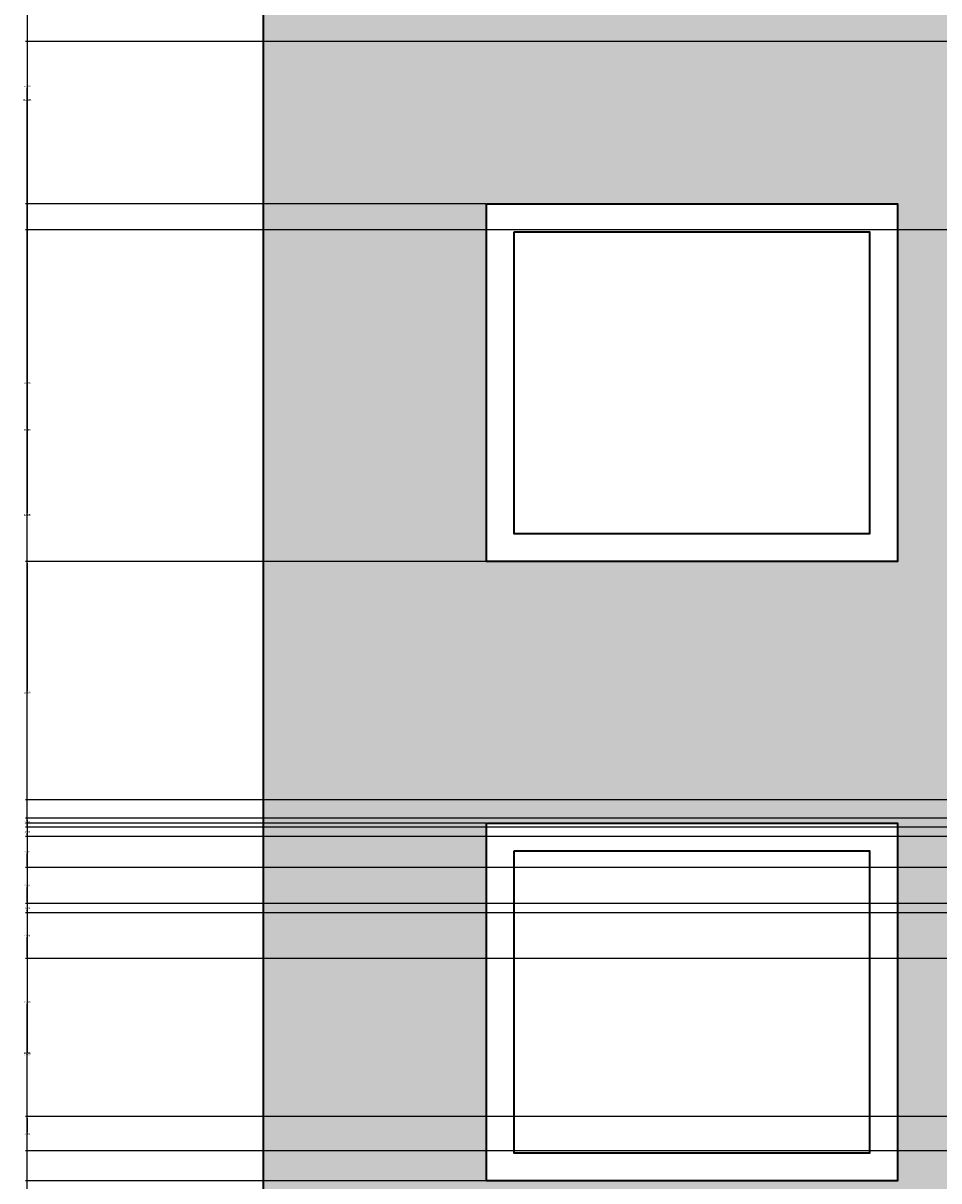
# Model space of a CAD drawing. Units: inches. Extents: x 93 to 565, y 123 to 656.
# Tile 5 of 18: x 93 to 192, y 324 to 450. Entities that reach past the tile are written whole.
import ezdxf

# ---------------------------------------------------------------- set-up
doc = ezdxf.new("R2010")
doc.units = ezdxf.units.IN
doc.header["$MEASUREMENT"] = 0
for name, color, linetype, lineweight in [('A-ANNO-DIMS', 2, 'Continuous', 18), ('A-ELEV', 7, 'Continuous', 35), ('A-WALL-PATT', 8, 'Continuous', 13)]:
    doc.layers.add(name, color=color, linetype=linetype, lineweight=lineweight)
doc.styles.get("Standard").update_dxf_attribs({"font": 'arial.ttf'})
doc.dimstyles.get("Standard").update_dxf_attribs({"dimtxt": 0.18, "dimasz": 0.18, "dimexe": 0.18, "dimexo": 0.0625, "dimgap": 0.09, "dimtad": 0, "dimtih": 1, "dimtoh": 1, "dimdec": 4, "dimzin": 0, "dimdsep": 46, "dimtxsty": 'Standard', "dimcen": 0.09, "dimadec": 0, "dimazin": 0, "dimtfac": 1, "dimtdec": 4, "dimtofl": 0, "dimtmove": 0, "dimatfit": 3, "dimfxl": 1, "dimtolj": 1, "dimtzin": 0, "dimarcsym": 0})

# ---------------------------------------------------------------- blocks, each defined once
blk = doc.blocks.new('*D27')
at = {"layer": 'A-ANNO-DIMS', "color": 0, "lineweight": -2, "transparency": 16777216}
for p, q in [((210.54, 519.04), (210.54, 134)), ((119.08, 159.67), (119.08, 134)), ((119.26, 134.18), (164.42, 134.18)), ((210.36, 134.18), (165.21, 134.18))]:
    blk.add_line(p, q, dxfattribs=at)
at = {"layer": 'A-ANNO-DIMS', "color": 0, "transparency": 16777216}
for points in [[(119.26, 134.21), (119.26, 134.15), (119.08, 134.18)], [(210.36, 134.21), (210.36, 134.15), (210.54, 134.18)]]:
    blk.add_solid(points, dxfattribs=at)
at = {"layer": 'Defpoints', "color": 0, "transparency": 16777216}
for p in [(210.54, 519.1), (119.08, 159.73), (210.54, 134.18)]:
    blk.add_point(p, dxfattribs=at)
at = {"layer": 'A-ANNO-DIMS', "color": 0, "transparency": 16777216, "insert": (164.81, 134.18), "char_height": 0.18, "attachment_point": 5}
blk.add_mtext('\\A1;91.46', dxfattribs=at)
blk = doc.blocks.new('*D31')
at = {"layer": 'A-ANNO-DIMS', "color": 0, "lineweight": -2, "transparency": 16777216}
for p, q in [((417.87, 630.4), (564.81, 630.4)), ((564.63, 630.22), (564.63, 395.25)), ((564.63, 159.91), (564.63, 394.89)), ((119.14, 159.73), (564.81, 159.73))]:
    blk.add_line(p, q, dxfattribs=at)
at = {"layer": 'A-ANNO-DIMS', "color": 0, "transparency": 16777216}
for points in [[(564.6, 630.22), (564.66, 630.22), (564.63, 630.4)], [(564.6, 159.91), (564.66, 159.91), (564.63, 159.73)]]:
    blk.add_solid(points, dxfattribs=at)
at = {"layer": 'Defpoints', "color": 0, "transparency": 16777216}
for p in [(417.81, 630.4), (564.63, 630.4), (119.08, 159.73)]:
    blk.add_point(p, dxfattribs=at)
at = {"layer": 'A-ANNO-DIMS', "color": 0, "transparency": 16777216, "insert": (564.63, 395.07), "char_height": 0.18, "attachment_point": 5}
blk.add_mtext('\\A1;470.7', dxfattribs=at)
blk = doc.blocks.new('*D34')
at = {"layer": 'A-ANNO-DIMS', "color": 0, "lineweight": -2, "transparency": 16777216}
for p, q in [((286.62, 363.73), (93.35, 363.73)), ((93.53, 363.55), (93.53, 338.52)), ((93.53, 313.13), (93.53, 338.16)), ((286.62, 312.95), (93.35, 312.95))]:
    blk.add_line(p, q, dxfattribs=at)
at = {"layer": 'A-ANNO-DIMS', "color": 0, "transparency": 16777216}
for points in [[(93.5, 363.55), (93.56, 363.55), (93.53, 363.73)], [(93.5, 313.13), (93.56, 313.13), (93.53, 312.95)]]:
    blk.add_solid(points, dxfattribs=at)
at = {"layer": 'Defpoints', "color": 0, "transparency": 16777216}
for p in [(93.53, 363.73), (286.69, 363.73), (286.69, 312.95)]:
    blk.add_point(p, dxfattribs=at)
at = {"layer": 'A-ANNO-DIMS', "color": 0, "transparency": 16777216, "insert": (93.53, 338.34), "char_height": 0.18, "attachment_point": 5}
blk.add_mtext('\\A1;50.78', dxfattribs=at)
blk = doc.blocks.new('*D35')
at = {"layer": 'A-ANNO-DIMS', "color": 0, "lineweight": -2, "transparency": 16777216}
for p, q in [((119.02, 519.1), (93.35, 519.1)), ((93.53, 518.92), (93.53, 441.6)), ((93.53, 363.91), (93.53, 441.23)), ((286.62, 363.73), (93.35, 363.73))]:
    blk.add_line(p, q, dxfattribs=at)
at = {"layer": 'A-ANNO-DIMS', "color": 0, "transparency": 16777216}
for points in [[(93.5, 518.92), (93.56, 518.92), (93.53, 519.1)], [(93.5, 363.91), (93.56, 363.91), (93.53, 363.73)]]:
    blk.add_solid(points, dxfattribs=at)
at = {"layer": 'Defpoints', "color": 0, "transparency": 16777216}
for p in [(93.53, 519.1), (119.08, 519.1), (286.69, 363.73)]:
    blk.add_point(p, dxfattribs=at)
at = {"layer": 'A-ANNO-DIMS', "color": 0, "transparency": 16777216, "insert": (93.53, 441.42), "char_height": 0.18, "attachment_point": 5}
blk.add_mtext('\\A1;155.37', dxfattribs=at)
blk = doc.blocks.new('*D43')
at = {"layer": 'A-ANNO-DIMS', "color": 0, "lineweight": -2, "transparency": 16777216}
for p, q in [((143.15, 363.17), (93.35, 363.17)), ((93.53, 362.99), (93.53, 344.01)), ((93.53, 324.67), (93.53, 343.65)), ((143.15, 324.49), (93.35, 324.49))]:
    blk.add_line(p, q, dxfattribs=at)
at = {"layer": 'A-ANNO-DIMS', "color": 0, "transparency": 16777216}
for points in [[(93.5, 362.99), (93.56, 362.99), (93.53, 363.17)], [(93.5, 324.67), (93.56, 324.67), (93.53, 324.49)]]:
    blk.add_solid(points, dxfattribs=at)
at = {"layer": 'Defpoints', "color": 0, "transparency": 16777216}
for p in [(93.53, 363.17), (143.21, 363.17), (143.21, 324.49)]:
    blk.add_point(p, dxfattribs=at)
at = {"layer": 'A-ANNO-DIMS', "color": 0, "transparency": 16777216, "insert": (93.53, 343.83), "char_height": 0.18, "attachment_point": 5}
blk.add_mtext('\\A1;38.685', dxfattribs=at)
blk = doc.blocks.new('*D44')
at = {"layer": 'A-ANNO-DIMS', "color": 0, "lineweight": -2, "transparency": 16777216}
for p, q in [((143.15, 391.47), (93.35, 391.47)), ((93.53, 391.29), (93.53, 377.5)), ((93.53, 363.35), (93.53, 377.14)), ((143.15, 363.17), (93.35, 363.17))]:
    blk.add_line(p, q, dxfattribs=at)
at = {"layer": 'A-ANNO-DIMS', "color": 0, "transparency": 16777216}
for points in [[(93.5, 391.29), (93.56, 391.29), (93.53, 391.47)], [(93.5, 363.35), (93.56, 363.35), (93.53, 363.17)]]:
    blk.add_solid(points, dxfattribs=at)
at = {"layer": 'Defpoints', "color": 0, "transparency": 16777216}
for p in [(93.53, 391.47), (143.21, 391.47), (143.21, 363.17)]:
    blk.add_point(p, dxfattribs=at)
at = {"layer": 'A-ANNO-DIMS', "color": 0, "transparency": 16777216, "insert": (93.53, 377.32), "char_height": 0.18, "attachment_point": 5}
blk.add_mtext('\\A1;28.295', dxfattribs=at)
blk = doc.blocks.new('*D45')
at = {"layer": 'A-ANNO-DIMS', "color": 0, "lineweight": -2, "transparency": 16777216}
for p, q in [((143.15, 430.15), (93.35, 430.15)), ((93.53, 429.97), (93.53, 410.99)), ((93.53, 391.65), (93.53, 410.63)), ((143.15, 391.47), (93.35, 391.47))]:
    blk.add_line(p, q, dxfattribs=at)
at = {"layer": 'A-ANNO-DIMS', "color": 0, "transparency": 16777216}
for points in [[(93.5, 429.97), (93.56, 429.97), (93.53, 430.15)], [(93.5, 391.65), (93.56, 391.65), (93.53, 391.47)]]:
    blk.add_solid(points, dxfattribs=at)
at = {"layer": 'Defpoints', "color": 0, "transparency": 16777216}
for p in [(93.53, 430.15), (143.21, 430.15), (143.21, 391.47)]:
    blk.add_point(p, dxfattribs=at)
at = {"layer": 'A-ANNO-DIMS', "color": 0, "transparency": 16777216, "insert": (93.53, 410.81), "char_height": 0.18, "attachment_point": 5}
blk.add_mtext('\\A1;38.685', dxfattribs=at)
blk = doc.blocks.new('*D46')
at = {"layer": 'A-ANNO-DIMS', "color": 0, "lineweight": -2, "transparency": 16777216}
for p, q in [((143.15, 455.66), (93.35, 455.66)), ((93.53, 455.48), (93.53, 443.09)), ((93.53, 430.33), (93.53, 442.72)), ((143.15, 430.15), (93.35, 430.15))]:
    blk.add_line(p, q, dxfattribs=at)
at = {"layer": 'A-ANNO-DIMS', "color": 0, "transparency": 16777216}
for points in [[(93.5, 455.48), (93.56, 455.48), (93.53, 455.66)], [(93.5, 430.33), (93.56, 430.33), (93.53, 430.15)]]:
    blk.add_solid(points, dxfattribs=at)
at = {"layer": 'Defpoints', "color": 0, "transparency": 16777216}
for p in [(93.53, 455.66), (143.21, 455.66), (143.21, 430.15)]:
    blk.add_point(p, dxfattribs=at)
at = {"layer": 'A-ANNO-DIMS', "color": 0, "transparency": 16777216, "insert": (93.53, 442.9), "char_height": 0.18, "attachment_point": 5}
blk.add_mtext('\\A1;25.507', dxfattribs=at)
blk = doc.blocks.new('*D65')
at = {"layer": 'A-ANNO-DIMS', "color": 0, "lineweight": -2, "transparency": 16777216}
for p, q in [((265.15, 427.35), (93.35, 427.35)), ((93.53, 427.17), (93.53, 396.71)), ((93.53, 365.89), (93.53, 396.35)), ((262.24, 365.71), (93.35, 365.71))]:
    blk.add_line(p, q, dxfattribs=at)
at = {"layer": 'A-ANNO-DIMS', "color": 0, "transparency": 16777216}
for points in [[(93.5, 427.17), (93.56, 427.17), (93.53, 427.35)], [(93.5, 365.89), (93.56, 365.89), (93.53, 365.71)]]:
    blk.add_solid(points, dxfattribs=at)
at = {"layer": 'Defpoints', "color": 0, "transparency": 16777216}
for p in [(93.53, 427.35), (265.21, 427.35), (262.3, 365.71)]:
    blk.add_point(p, dxfattribs=at)
at = {"layer": 'A-ANNO-DIMS', "color": 0, "transparency": 16777216, "insert": (93.53, 396.53), "char_height": 0.18, "attachment_point": 5}
blk.add_mtext('\\A1;61.64', dxfattribs=at)
blk = doc.blocks.new('*D72')
at = {"layer": 'A-ANNO-DIMS', "color": 0, "lineweight": -2, "transparency": 16777216}
for p, q in [((295.62, 447.73), (93.35, 447.73)), ((93.53, 447.55), (93.53, 405.91)), ((93.53, 363.91), (93.53, 405.55)), ((286.62, 363.73), (93.35, 363.73))]:
    blk.add_line(p, q, dxfattribs=at)
at = {"layer": 'A-ANNO-DIMS', "color": 0, "transparency": 16777216}
for points in [[(93.5, 447.55), (93.56, 447.55), (93.53, 447.73)], [(93.5, 363.91), (93.56, 363.91), (93.53, 363.73)]]:
    blk.add_solid(points, dxfattribs=at)
at = {"layer": 'Defpoints', "color": 0, "transparency": 16777216}
for p in [(295.69, 447.73), (93.53, 363.73), (286.69, 363.73)]:
    blk.add_point(p, dxfattribs=at)
at = {"layer": 'A-ANNO-DIMS', "color": 0, "transparency": 16777216, "insert": (93.53, 405.73), "char_height": 0.18, "attachment_point": 5}
blk.add_mtext('\\A1;84', dxfattribs=at)
blk = doc.blocks.new('*D106')
at = {"layer": 'A-ANNO-DIMS', "color": 0, "lineweight": -2, "transparency": 16777216}
for p, q in [((210.54, 519.04), (210.54, 134)), ((119.08, 159.67), (119.08, 134)), ((119.26, 134.18), (164.35, 134.18)), ((210.36, 134.18), (165.28, 134.18))]:
    blk.add_line(p, q, dxfattribs=at)
at = {"layer": 'A-ANNO-DIMS', "color": 0, "transparency": 16777216}
for points in [[(119.26, 134.21), (119.26, 134.15), (119.08, 134.18)], [(210.36, 134.21), (210.36, 134.15), (210.54, 134.18)]]:
    blk.add_solid(points, dxfattribs=at)
at = {"layer": 'Defpoints', "color": 0, "transparency": 16777216}
for p in [(210.54, 519.1), (119.08, 159.73), (210.54, 134.18)]:
    blk.add_point(p, dxfattribs=at)
at = {"layer": 'A-ANNO-DIMS', "color": 0, "transparency": 16777216, "insert": (164.81, 134.18), "char_height": 0.18, "attachment_point": 5}
blk.add_mtext('\\A1;91.465', dxfattribs=at)
blk = doc.blocks.new('*D110')
at = {"layer": 'A-ANNO-DIMS', "color": 0, "lineweight": -2, "transparency": 16777216}
for p, q in [((417.87, 630.4), (564.81, 630.4)), ((564.63, 630.22), (564.63, 395.25)), ((564.63, 159.91), (564.63, 394.89)), ((119.14, 159.73), (564.81, 159.73))]:
    blk.add_line(p, q, dxfattribs=at)
at = {"layer": 'A-ANNO-DIMS', "color": 0, "transparency": 16777216}
for points in [[(564.6, 630.22), (564.66, 630.22), (564.63, 630.4)], [(564.6, 159.91), (564.66, 159.91), (564.63, 159.73)]]:
    blk.add_solid(points, dxfattribs=at)
at = {"layer": 'Defpoints', "color": 0, "transparency": 16777216}
for p in [(417.81, 630.4), (564.63, 630.4), (119.08, 159.73)]:
    blk.add_point(p, dxfattribs=at)
at = {"layer": 'A-ANNO-DIMS', "color": 0, "transparency": 16777216, "insert": (564.63, 395.07), "char_height": 0.18, "attachment_point": 5}
blk.add_mtext('\\A1;470.673', dxfattribs=at)
blk = doc.blocks.new('*D113')
at = {"layer": 'A-ANNO-DIMS', "color": 0, "lineweight": -2, "transparency": 16777216}
for p, q in [((286.62, 363.73), (93.35, 363.73)), ((93.53, 363.55), (93.53, 338.52)), ((93.53, 313.13), (93.53, 338.16)), ((286.62, 312.95), (93.35, 312.95))]:
    blk.add_line(p, q, dxfattribs=at)
at = {"layer": 'A-ANNO-DIMS', "color": 0, "transparency": 16777216}
for points in [[(93.5, 363.55), (93.56, 363.55), (93.53, 363.73)], [(93.5, 313.13), (93.56, 313.13), (93.53, 312.95)]]:
    blk.add_solid(points, dxfattribs=at)
at = {"layer": 'Defpoints', "color": 0, "transparency": 16777216}
for p in [(93.53, 363.73), (286.69, 363.73), (286.69, 312.95)]:
    blk.add_point(p, dxfattribs=at)
at = {"layer": 'A-ANNO-DIMS', "color": 0, "transparency": 16777216, "insert": (93.53, 338.34), "char_height": 0.18, "attachment_point": 5}
blk.add_mtext('\\A1;50.783', dxfattribs=at)
blk = doc.blocks.new('*D114')
at = {"layer": 'A-ANNO-DIMS', "color": 0, "lineweight": -2, "transparency": 16777216}
for p, q in [((119.02, 519.1), (93.35, 519.1)), ((93.53, 518.92), (93.53, 441.6)), ((93.53, 363.91), (93.53, 441.23)), ((286.62, 363.73), (93.35, 363.73))]:
    blk.add_line(p, q, dxfattribs=at)
at = {"layer": 'A-ANNO-DIMS', "color": 0, "transparency": 16777216}
for points in [[(93.5, 518.92), (93.56, 518.92), (93.53, 519.1)], [(93.5, 363.91), (93.56, 363.91), (93.53, 363.73)]]:
    blk.add_solid(points, dxfattribs=at)
at = {"layer": 'Defpoints', "color": 0, "transparency": 16777216}
for p in [(93.53, 519.1), (119.08, 519.1), (286.69, 363.73)]:
    blk.add_point(p, dxfattribs=at)
at = {"layer": 'A-ANNO-DIMS', "color": 0, "transparency": 16777216, "insert": (93.53, 441.42), "char_height": 0.18, "attachment_point": 5}
blk.add_mtext('\\A1;155.368', dxfattribs=at)
blk = doc.blocks.new('*D122')
at = {"layer": 'A-ANNO-DIMS', "color": 0, "lineweight": -2, "transparency": 16777216}
for p, q in [((143.15, 363.17), (93.35, 363.17)), ((93.53, 362.99), (93.53, 344.01)), ((93.53, 324.67), (93.53, 343.65)), ((143.15, 324.49), (93.35, 324.49))]:
    blk.add_line(p, q, dxfattribs=at)
at = {"layer": 'A-ANNO-DIMS', "color": 0, "transparency": 16777216}
for points in [[(93.5, 362.99), (93.56, 362.99), (93.53, 363.17)], [(93.5, 324.67), (93.56, 324.67), (93.53, 324.49)]]:
    blk.add_solid(points, dxfattribs=at)
at = {"layer": 'Defpoints', "color": 0, "transparency": 16777216}
for p in [(93.53, 363.17), (143.21, 363.17), (143.21, 324.49)]:
    blk.add_point(p, dxfattribs=at)
at = {"layer": 'A-ANNO-DIMS', "color": 0, "transparency": 16777216, "insert": (93.53, 343.83), "char_height": 0.18, "attachment_point": 5}
blk.add_mtext('\\A1;38.685', dxfattribs=at)
blk = doc.blocks.new('*D123')
at = {"layer": 'A-ANNO-DIMS', "color": 0, "lineweight": -2, "transparency": 16777216}
for p, q in [((143.15, 391.47), (93.35, 391.47)), ((93.53, 391.29), (93.53, 377.5)), ((93.53, 363.35), (93.53, 377.14)), ((143.15, 363.17), (93.35, 363.17))]:
    blk.add_line(p, q, dxfattribs=at)
at = {"layer": 'A-ANNO-DIMS', "color": 0, "transparency": 16777216}
for points in [[(93.5, 391.29), (93.56, 391.29), (93.53, 391.47)], [(93.5, 363.35), (93.56, 363.35), (93.53, 363.17)]]:
    blk.add_solid(points, dxfattribs=at)
at = {"layer": 'Defpoints', "color": 0, "transparency": 16777216}
for p in [(93.53, 391.47), (143.21, 391.47), (143.21, 363.17)]:
    blk.add_point(p, dxfattribs=at)
at = {"layer": 'A-ANNO-DIMS', "color": 0, "transparency": 16777216, "insert": (93.53, 377.32), "char_height": 0.18, "attachment_point": 5}
blk.add_mtext('\\A1;28.295', dxfattribs=at)
blk = doc.blocks.new('*D124')
at = {"layer": 'A-ANNO-DIMS', "color": 0, "lineweight": -2, "transparency": 16777216}
for p, q in [((143.15, 430.15), (93.35, 430.15)), ((93.53, 429.97), (93.53, 410.99)), ((93.53, 391.65), (93.53, 410.63)), ((143.15, 391.47), (93.35, 391.47))]:
    blk.add_line(p, q, dxfattribs=at)
at = {"layer": 'A-ANNO-DIMS', "color": 0, "transparency": 16777216}
for points in [[(93.5, 429.97), (93.56, 429.97), (93.53, 430.15)], [(93.5, 391.65), (93.56, 391.65), (93.53, 391.47)]]:
    blk.add_solid(points, dxfattribs=at)
at = {"layer": 'Defpoints', "color": 0, "transparency": 16777216}
for p in [(93.53, 430.15), (143.21, 430.15), (143.21, 391.47)]:
    blk.add_point(p, dxfattribs=at)
at = {"layer": 'A-ANNO-DIMS', "color": 0, "transparency": 16777216, "insert": (93.53, 410.81), "char_height": 0.18, "attachment_point": 5}
blk.add_mtext('\\A1;38.685', dxfattribs=at)
blk = doc.blocks.new('*D125')
at = {"layer": 'A-ANNO-DIMS', "color": 0, "lineweight": -2, "transparency": 16777216}
for p, q in [((143.15, 455.66), (93.35, 455.66)), ((93.53, 455.48), (93.53, 443.09)), ((93.53, 430.33), (93.53, 442.72)), ((143.15, 430.15), (93.35, 430.15))]:
    blk.add_line(p, q, dxfattribs=at)
at = {"layer": 'A-ANNO-DIMS', "color": 0, "transparency": 16777216}
for points in [[(93.5, 455.48), (93.56, 455.48), (93.53, 455.66)], [(93.5, 430.33), (93.56, 430.33), (93.53, 430.15)]]:
    blk.add_solid(points, dxfattribs=at)
at = {"layer": 'Defpoints', "color": 0, "transparency": 16777216}
for p in [(93.53, 455.66), (143.21, 455.66), (143.21, 430.15)]:
    blk.add_point(p, dxfattribs=at)
at = {"layer": 'A-ANNO-DIMS', "color": 0, "transparency": 16777216, "insert": (93.53, 442.9), "char_height": 0.18, "attachment_point": 5}
blk.add_mtext('\\A1;25.507', dxfattribs=at)
blk = doc.blocks.new('*D144')
at = {"layer": 'A-ANNO-DIMS', "color": 0, "lineweight": -2, "transparency": 16777216}
for p, q in [((265.15, 427.35), (93.35, 427.35)), ((93.53, 427.17), (93.53, 396.71)), ((93.53, 365.89), (93.53, 396.35)), ((262.24, 365.71), (93.35, 365.71))]:
    blk.add_line(p, q, dxfattribs=at)
at = {"layer": 'A-ANNO-DIMS', "color": 0, "transparency": 16777216}
for points in [[(93.5, 427.17), (93.56, 427.17), (93.53, 427.35)], [(93.5, 365.89), (93.56, 365.89), (93.53, 365.71)]]:
    blk.add_solid(points, dxfattribs=at)
at = {"layer": 'Defpoints', "color": 0, "transparency": 16777216}
for p in [(93.53, 427.35), (265.21, 427.35), (262.3, 365.71)]:
    blk.add_point(p, dxfattribs=at)
at = {"layer": 'A-ANNO-DIMS', "color": 0, "transparency": 16777216, "insert": (93.53, 396.53), "char_height": 0.18, "attachment_point": 5}
blk.add_mtext('\\A1;61.638', dxfattribs=at)
blk = doc.blocks.new('*D151')
at = {"layer": 'A-ANNO-DIMS', "color": 0, "lineweight": -2, "transparency": 16777216}
for p, q in [((295.62, 447.73), (93.35, 447.73)), ((93.53, 447.55), (93.53, 405.91)), ((93.53, 363.91), (93.53, 405.55)), ((286.62, 363.73), (93.35, 363.73))]:
    blk.add_line(p, q, dxfattribs=at)
at = {"layer": 'A-ANNO-DIMS', "color": 0, "transparency": 16777216}
for points in [[(93.5, 447.55), (93.56, 447.55), (93.53, 447.73)], [(93.5, 363.91), (93.56, 363.91), (93.53, 363.73)]]:
    blk.add_solid(points, dxfattribs=at)
at = {"layer": 'Defpoints', "color": 0, "transparency": 16777216}
for p in [(295.69, 447.73), (93.53, 363.73), (286.69, 363.73)]:
    blk.add_point(p, dxfattribs=at)
at = {"layer": 'A-ANNO-DIMS', "color": 0, "transparency": 16777216, "insert": (93.53, 405.73), "char_height": 0.18, "attachment_point": 5}
blk.add_mtext('\\A1;84.000', dxfattribs=at)
blk = doc.blocks.new('*D190')
at = {"layer": 'A-ANNO-DIMS', "color": 0, "lineweight": -2, "transparency": 16777216}
for p, q in [((514.58, 348.55), (93.35, 348.55)), ((93.53, 348.37), (93.53, 338.33)), ((93.53, 327.91), (93.53, 337.96)), ((539.02, 327.73), (93.35, 327.73))]:
    blk.add_line(p, q, dxfattribs=at)
at = {"layer": 'A-ANNO-DIMS', "color": 0, "transparency": 16777216}
for points in [[(93.5, 348.37), (93.56, 348.37), (93.53, 348.55)], [(93.5, 327.91), (93.56, 327.91), (93.53, 327.73)]]:
    blk.add_solid(points, dxfattribs=at)
at = {"layer": 'Defpoints', "color": 0, "transparency": 16777216}
for p in [(93.53, 348.55), (514.64, 348.55), (539.08, 327.73)]:
    blk.add_point(p, dxfattribs=at)
at = {"layer": 'A-ANNO-DIMS', "color": 0, "transparency": 16777216, "insert": (93.53, 338.14), "char_height": 0.18, "attachment_point": 5}
blk.add_mtext('\\A1;20.822', dxfattribs=at)
blk = doc.blocks.new('*D191')
at = {"layer": 'A-ANNO-DIMS', "color": 0, "lineweight": -2, "transparency": 16777216}
for p, q in [((514.58, 353.47), (93.35, 353.47)), ((93.53, 353.29), (93.53, 351.2)), ((93.53, 348.73), (93.53, 350.83)), ((514.58, 348.55), (93.35, 348.55))]:
    blk.add_line(p, q, dxfattribs=at)
at = {"layer": 'A-ANNO-DIMS', "color": 0, "transparency": 16777216}
for points in [[(93.5, 353.29), (93.56, 353.29), (93.53, 353.47)], [(93.5, 348.73), (93.56, 348.73), (93.53, 348.55)]]:
    blk.add_solid(points, dxfattribs=at)
at = {"layer": 'Defpoints', "color": 0, "transparency": 16777216}
for p in [(93.53, 353.47), (514.64, 353.47), (514.64, 348.55)]:
    blk.add_point(p, dxfattribs=at)
at = {"layer": 'A-ANNO-DIMS', "color": 0, "transparency": 16777216, "insert": (93.53, 351.01), "char_height": 0.18, "attachment_point": 5}
blk.add_mtext('\\A1;4.918', dxfattribs=at)
blk = doc.blocks.new('*D192')
at = {"layer": 'A-ANNO-DIMS', "color": 0, "lineweight": -2, "transparency": 16777216}
for p, q in [((514.58, 354.47), (93.35, 354.47)), ((514.58, 353.47), (93.35, 353.47)), ((93.53, 354.29), (93.53, 354.15)), ((93.53, 353.65), (93.53, 353.79))]:
    blk.add_line(p, q, dxfattribs=at)
at = {"layer": 'A-ANNO-DIMS', "color": 0, "transparency": 16777216}
for points in [[(93.5, 354.29), (93.56, 354.29), (93.53, 354.47)], [(93.5, 353.65), (93.56, 353.65), (93.53, 353.47)]]:
    blk.add_solid(points, dxfattribs=at)
at = {"layer": 'Defpoints', "color": 0, "transparency": 16777216}
for p in [(93.53, 354.47), (514.64, 354.47), (514.64, 353.47)]:
    blk.add_point(p, dxfattribs=at)
at = {"layer": 'A-ANNO-DIMS', "color": 0, "transparency": 16777216, "insert": (93.53, 353.97), "char_height": 0.18, "attachment_point": 5}
blk.add_mtext('\\A1;1.000', dxfattribs=at)
blk = doc.blocks.new('*D193')
at = {"layer": 'A-ANNO-DIMS', "color": 0, "lineweight": -2, "transparency": 16777216}
for p, q in [((514.58, 358.37), (93.35, 358.37)), ((93.53, 358.19), (93.53, 356.61)), ((93.53, 354.65), (93.53, 356.24)), ((514.58, 354.47), (93.35, 354.47))]:
    blk.add_line(p, q, dxfattribs=at)
at = {"layer": 'A-ANNO-DIMS', "color": 0, "transparency": 16777216}
for points in [[(93.5, 358.19), (93.56, 358.19), (93.53, 358.37)], [(93.5, 354.65), (93.56, 354.65), (93.53, 354.47)]]:
    blk.add_solid(points, dxfattribs=at)
at = {"layer": 'Defpoints', "color": 0, "transparency": 16777216}
for p in [(93.53, 358.37), (514.64, 358.37), (514.64, 354.47)]:
    blk.add_point(p, dxfattribs=at)
at = {"layer": 'A-ANNO-DIMS', "color": 0, "transparency": 16777216, "insert": (93.53, 356.42), "char_height": 0.18, "attachment_point": 5}
blk.add_mtext('\\A1;3.901', dxfattribs=at)
blk = doc.blocks.new('*D194')
at = {"layer": 'A-ANNO-DIMS', "color": 0, "lineweight": -2, "transparency": 16777216}
for p, q in [((524.92, 361.75), (93.35, 361.75)), ((93.53, 361.57), (93.53, 360.24)), ((93.53, 358.55), (93.53, 359.88)), ((514.58, 358.37), (93.35, 358.37))]:
    blk.add_line(p, q, dxfattribs=at)
at = {"layer": 'A-ANNO-DIMS', "color": 0, "transparency": 16777216}
for points in [[(93.5, 361.57), (93.56, 361.57), (93.53, 361.75)], [(93.5, 358.55), (93.56, 358.55), (93.53, 358.37)]]:
    blk.add_solid(points, dxfattribs=at)
at = {"layer": 'Defpoints', "color": 0, "transparency": 16777216}
for p in [(93.53, 361.75), (524.99, 361.75), (514.64, 358.37)]:
    blk.add_point(p, dxfattribs=at)
at = {"layer": 'A-ANNO-DIMS', "color": 0, "transparency": 16777216, "insert": (93.53, 360.06), "char_height": 0.18, "attachment_point": 5}
blk.add_mtext('\\A1;3.374', dxfattribs=at)
blk = doc.blocks.new('*D195')
at = {"layer": 'A-ANNO-DIMS', "color": 0, "lineweight": -2, "transparency": 16777216}
for p, q in [((524.92, 362.75), (93.35, 362.75)), ((93.53, 362.57), (93.53, 362.43)), ((93.53, 361.93), (93.53, 362.07)), ((524.92, 361.75), (93.35, 361.75))]:
    blk.add_line(p, q, dxfattribs=at)
at = {"layer": 'A-ANNO-DIMS', "color": 0, "transparency": 16777216}
for points in [[(93.5, 362.57), (93.56, 362.57), (93.53, 362.75)], [(93.5, 361.93), (93.56, 361.93), (93.53, 361.75)]]:
    blk.add_solid(points, dxfattribs=at)
at = {"layer": 'Defpoints', "color": 0, "transparency": 16777216}
for p in [(93.53, 362.75), (524.99, 362.75), (524.99, 361.75)]:
    blk.add_point(p, dxfattribs=at)
at = {"layer": 'A-ANNO-DIMS', "color": 0, "transparency": 16777216, "insert": (93.53, 362.25), "char_height": 0.18, "attachment_point": 5}
blk.add_mtext('\\A1;1.000', dxfattribs=at)
blk = doc.blocks.new('*D196')
at = {"layer": 'A-ANNO-DIMS', "color": 0, "lineweight": -2, "transparency": 16777216}
for p, q in [((524.92, 363.73), (93.35, 363.73)), ((93.53, 363.55), (93.53, 363.42)), ((524.92, 362.75), (93.35, 362.75)), ((93.53, 362.93), (93.53, 363.06))]:
    blk.add_line(p, q, dxfattribs=at)
at = {"layer": 'A-ANNO-DIMS', "color": 0, "transparency": 16777216}
for points in [[(93.5, 363.55), (93.56, 363.55), (93.53, 363.73)], [(93.5, 362.93), (93.56, 362.93), (93.53, 362.75)]]:
    blk.add_solid(points, dxfattribs=at)
at = {"layer": 'Defpoints', "color": 0, "transparency": 16777216}
for p in [(93.53, 363.73), (524.99, 363.73), (524.99, 362.75)]:
    blk.add_point(p, dxfattribs=at)
at = {"layer": 'A-ANNO-DIMS', "color": 0, "transparency": 16777216, "insert": (93.53, 363.24), "char_height": 0.18, "attachment_point": 5}
blk.add_mtext('\\A1;0.985', dxfattribs=at)
blk = doc.blocks.new('*D198')
at = {"layer": 'A-ANNO-DIMS', "color": 0, "lineweight": -2, "transparency": 16777216}
for p, q in [((515.95, 331.43), (93.35, 331.43)), ((93.53, 331.25), (93.53, 329.76)), ((93.53, 327.91), (93.53, 329.4)), ((539.02, 327.73), (93.35, 327.73))]:
    blk.add_line(p, q, dxfattribs=at)
at = {"layer": 'A-ANNO-DIMS', "color": 0, "transparency": 16777216}
for points in [[(93.5, 331.25), (93.56, 331.25), (93.53, 331.43)], [(93.5, 327.91), (93.56, 327.91), (93.53, 327.73)]]:
    blk.add_solid(points, dxfattribs=at)
at = {"layer": 'Defpoints', "color": 0, "transparency": 16777216}
for p in [(93.53, 331.43), (516.01, 331.43), (539.08, 327.73)]:
    blk.add_point(p, dxfattribs=at)
at = {"layer": 'A-ANNO-DIMS', "color": 0, "transparency": 16777216, "insert": (93.53, 329.58), "char_height": 0.18, "attachment_point": 5}
blk.add_mtext('\\A1;3.701', dxfattribs=at)

msp = doc.modelspace()

# ---------------------------------------------------------------- hatches: boundary and pattern name
at = {"layer": 'A-WALL-PATT'}
h = msp.add_hatch(dxfattribs=at)
h.set_pattern_fill('STARS', color=256, scale=21)
h.paths.add_polyline_path([(210.5443, 507.7323), (210.5443, 519.0999), (119.0794, 519.0999), (119.0794, 507.7323), (119.0794, 183.7323), (210.5443, 183.7323)])
h.paths.add_polyline_path([(187.648, 430.1508), (187.648, 391.4653), (143.2118, 391.4653), (143.2118, 430.1508)], flags=16)
h.paths.add_polyline_path([(187.648, 455.6579), (143.2118, 455.6579), (143.2118, 494.3434), (187.648, 494.3434)], flags=16)
h.paths.add_polyline_path([(184.648, 427.1508), (184.648, 394.4653), (146.2118, 394.4653), (146.2118, 427.1508)], flags=0)
h.paths.add_polyline_path([(184.648, 458.6579), (146.2118, 458.6579), (146.2118, 491.3434), (184.648, 491.3434)], flags=0)
h.paths.add_polyline_path([(187.648, 363.1705), (187.648, 324.485), (143.2118, 324.485), (143.2118, 363.1705)], flags=16)
h.paths.add_polyline_path([(184.648, 360.1705), (184.648, 327.485), (146.2118, 327.485), (146.2118, 360.1705)], flags=0)
h.paths.add_polyline_path([(187.648, 300.3249), (187.648, 261.6394), (143.2118, 261.6394), (143.2118, 300.3249)], flags=16)
h.paths.add_polyline_path([(184.648, 297.3249), (184.648, 264.6394), (146.2118, 264.6394), (146.2118, 297.3249)], flags=0)
h.paths.add_polyline_path([(187.648, 243.6441), (187.648, 204.9587), (143.2118, 204.9587), (143.2118, 243.6441)], flags=16)
h.paths.add_polyline_path([(184.648, 240.6441), (184.648, 207.9587), (146.2118, 207.9587), (146.2118, 240.6441)], flags=0)

# ---------------------------------------------------------------- linework, layer by layer
at = {"layer": 'A-ELEV'}
for p, q in [((119.0794, 183.7323), (119.0794, 507.7323)), ((119.0794, 327.7323), (119.0794, 339.7323))]:
    msp.add_line(p, q, dxfattribs=at)
for points in [[(143.2118, 430.1508), (187.648, 430.1508), (187.648, 391.4653), (143.2118, 391.4653)], [(146.2118, 427.1508), (184.648, 427.1508), (184.648, 394.4653), (146.2118, 394.4653)], [(143.2118, 363.1705), (187.648, 363.1705), (187.648, 324.485), (143.2118, 324.485)], [(146.2118, 360.1705), (184.648, 360.1705), (184.648, 327.485), (146.2118, 327.485)]]:
    msp.add_lwpolyline(points, close=True, dxfattribs=at)

# ---------------------------------------------------------------- dimensions: what is measured, and where the dimension line sits
at = {"layer": 'A-ANNO-DIMS'}
for base, p1, p2, override, picture, middle in [((564.6294, 630.4048), (119.0794, 159.7323), (417.8097, 630.4048), {"dimdec": 1, "dimlfac": 1, "dimrnd": 0, "dimzin": 0, "dimdsep": 46, "dimlunit": 2}, '*D31', (564.6294, 395.0685)), ((564.62936, 630.40478), (119.07936, 159.73225), (417.80971, 630.40477), {"dimdec": 3, "dimlfac": 1, "dimrnd": 0, "dimzin": 0, "dimdsep": 46, "dimlunit": 2}, '*D110', (564.62936, 395.06851)), ((93.5294, 519.0999), (286.6874, 363.7323), (119.0794, 519.0999), {"dimdec": 3, "dimlfac": 1, "dimrnd": 0, "dimzin": 0, "dimdsep": 46, "dimlunit": 2}, '*D114', (93.5294, 441.4161)), ((93.5294, 519.0999), (286.6874, 363.7323), (119.0794, 519.0999), {"dimdec": 2, "dimlfac": 1, "dimrnd": 0, "dimzin": 0, "dimdsep": 46, "dimlunit": 2}, '*D35', (93.5294, 441.4161)), ((93.5294, 455.6579), (143.2118, 430.1508), (143.2118, 455.6579), {"dimdec": 3, "dimlfac": 1, "dimrnd": 0, "dimzin": 0, "dimdsep": 46, "dimlunit": 2}, '*D46', (93.5294, 442.9043)), ((93.5294, 455.6579), (143.2118, 430.1508), (143.2118, 455.6579), {"dimdec": 3, "dimlfac": 1, "dimrnd": 0, "dimzin": 0, "dimdsep": 46, "dimlunit": 2}, '*D125', (93.5294, 442.9043)), ((93.5294, 363.7323), (295.6874, 447.7323), (286.6874, 363.7323), {"dimdec": 3, "dimlfac": 1, "dimrnd": 0, "dimzin": 0, "dimdsep": 46, "dimlunit": 2}, '*D151', (93.5294, 405.7323)), ((93.5294, 363.7323), (295.6874, 447.7323), (286.6874, 363.7323), {"dimdec": 0, "dimlfac": 1, "dimrnd": 0, "dimzin": 0, "dimdsep": 46, "dimlunit": 2}, '*D72', (93.5294, 405.7323)), ((93.52936, 430.15075), (143.21177, 391.46529), (143.21177, 430.15075), {"dimdec": 3, "dimlfac": 1, "dimrnd": 0, "dimzin": 0, "dimdsep": 46, "dimlunit": 2}, '*D45', (93.52936, 410.80802)), ((93.52936, 430.15075), (143.21177, 391.46529), (143.21177, 430.15075), {"dimdec": 3, "dimlfac": 1, "dimrnd": 0, "dimzin": 0, "dimdsep": 46, "dimlunit": 2}, '*D124', (93.52936, 410.80802)), ((93.5294, 427.3478), (262.3003, 365.71), (265.2145, 427.3478), {"dimdec": 3, "dimlfac": 1, "dimrnd": 0, "dimzin": 0, "dimdsep": 46, "dimlunit": 2}, '*D144', (93.5294, 396.5289)), ((93.5294, 427.3478), (262.3003, 365.71), (265.2145, 427.3478), {"dimdec": 2, "dimlfac": 1, "dimrnd": 0, "dimzin": 0, "dimdsep": 46, "dimlunit": 2}, '*D65', (93.5294, 396.5289)), ((93.5294, 391.4653), (143.2118, 363.1705), (143.2118, 391.4653), {"dimdec": 3, "dimlfac": 1, "dimrnd": 0, "dimzin": 0, "dimdsep": 46, "dimlunit": 2}, '*D44', (93.5294, 377.3179)), ((93.5294, 391.4653), (143.2118, 363.1705), (143.2118, 391.4653), {"dimdec": 3, "dimlfac": 1, "dimrnd": 0, "dimzin": 0, "dimdsep": 46, "dimlunit": 2}, '*D123', (93.5294, 377.3179)), ((93.5294, 363.7323), (286.6874, 312.9491), (286.6874, 363.7323), {"dimdec": 3, "dimlfac": 1, "dimrnd": 0, "dimzin": 0, "dimdsep": 46, "dimlunit": 2}, '*D113', (93.5294, 338.3407)), ((93.52936, 363.17052), (143.21177, 324.48505), (143.21177, 363.17052), {"dimdec": 3, "dimlfac": 1, "dimrnd": 0, "dimzin": 0, "dimdsep": 46, "dimlunit": 2}, '*D43', (93.52936, 343.82778)), ((93.52936, 363.17052), (143.21177, 324.48505), (143.21177, 363.17052), {"dimdec": 3, "dimlfac": 1, "dimrnd": 0, "dimzin": 0, "dimdsep": 46, "dimlunit": 2}, '*D122', (93.52936, 343.82778)), ((93.5294, 363.7323), (286.6874, 312.9491), (286.6874, 363.7323), {"dimdec": 2, "dimlfac": 1, "dimrnd": 0, "dimzin": 0, "dimdsep": 46, "dimlunit": 2}, '*D34', (93.5294, 338.3407)), ((93.5294, 363.7323), (524.9864, 362.7477), (524.9864, 363.7323), {"dimdec": 3, "dimlfac": 1, "dimrnd": 0, "dimzin": 0, "dimdsep": 46, "dimlunit": 2}, '*D196', (93.5294, 363.24)), ((93.5294, 362.7477), (524.9864, 361.7477), (524.9864, 362.7477), {"dimdec": 3, "dimlfac": 1, "dimrnd": 0, "dimzin": 0, "dimdsep": 46, "dimlunit": 2}, '*D195', (93.5294, 362.2477)), ((93.5294, 361.7477), (514.6424, 358.3735), (524.9864, 361.7477), {"dimdec": 3, "dimlfac": 1, "dimrnd": 0, "dimzin": 0, "dimdsep": 46, "dimlunit": 2}, '*D194', (93.5294, 360.0606)), ((93.5294, 358.3735), (514.6424, 354.4729), (514.6424, 358.3735), {"dimdec": 3, "dimlfac": 1, "dimrnd": 0, "dimzin": 0, "dimdsep": 46, "dimlunit": 2}, '*D193', (93.5294, 356.4232)), ((93.5294, 354.4729), (514.6424, 353.4729), (514.6424, 354.4729), {"dimdec": 3, "dimlfac": 1, "dimrnd": 0, "dimzin": 0, "dimdsep": 46, "dimlunit": 2}, '*D192', (93.5294, 353.9729)), ((93.5294, 353.4729), (514.6424, 348.5546), (514.6424, 353.4729), {"dimdec": 3, "dimlfac": 1, "dimrnd": 0, "dimzin": 0, "dimdsep": 46, "dimlunit": 2}, '*D191', (93.5294, 351.0137)), ((93.5294, 348.5546), (539.0794, 327.7323), (514.6424, 348.5546), {"dimdec": 3, "dimlfac": 1, "dimrnd": 0, "dimzin": 0, "dimdsep": 46, "dimlunit": 2}, '*D190', (93.5294, 338.1434)), ((93.5294, 331.4335), (539.0794, 327.7323), (516.0099, 331.4335), {"dimdec": 3, "dimlfac": 1, "dimrnd": 0, "dimzin": 0, "dimdsep": 46, "dimlunit": 2}, '*D198', (93.5294, 329.5829))]:
    dim = msp.add_linear_dim(base=base, p1=p1, p2=p2, angle=90, dimstyle='Standard', override=override, dxfattribs=at)
    dim.commit()
    dim.dimension.update_dxf_attribs({"geometry": picture, "text_midpoint": middle})
for override, picture in [({"dimdec": 2, "dimlfac": 1, "dimrnd": 0, "dimzin": 0, "dimdsep": 46, "dimlunit": 2}, '*D27'), ({"dimdec": 3, "dimlfac": 1, "dimrnd": 0, "dimzin": 0, "dimdsep": 46, "dimlunit": 2}, '*D106')]:
    dim = msp.add_linear_dim(base=(210.5443, 134.1823), p1=(119.0794, 159.7323), p2=(210.5443, 519.0999), dimstyle='Standard', override=override, dxfattribs=at)
    dim.commit()
    dim.dimension.update_dxf_attribs({"geometry": picture, "text_midpoint": (164.8118, 134.1823)})

doc.saveas('drawing.dxf')
